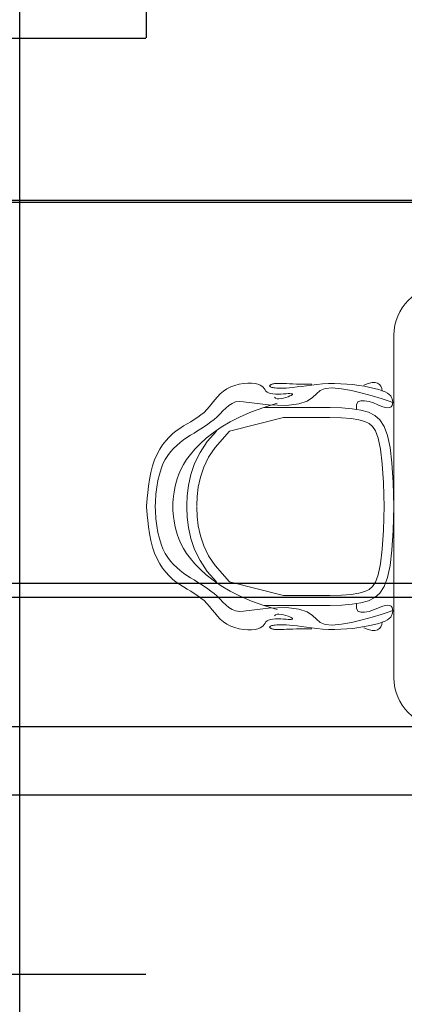
# Model space of a CAD drawing. Units: inches. Extents: x 1454 to 2136, y 626 to 1213.
# Tile 7 of 23: x 1561 to 1592, y 1062 to 1141. Entities that reach past the tile are written whole.
import ezdxf

# ---------------------------------------------------------------- set-up
doc = ezdxf.new("R2010")
doc.units = ezdxf.units.IN
doc.header["$MEASUREMENT"] = 0
for name, color, linetype, lineweight in [('A-ANNO-DIMS', 2, 'Continuous', 18), ('A-FURN-PATT', 252, 'Continuous', 13), ('conference', 41, 'Continuous', 18)]:
    doc.layers.add(name, color=color, linetype=linetype, lineweight=lineweight)
doc.styles.get("Standard").update_dxf_attribs({"font": 'arial.ttf'})
doc.dimstyles.get("Standard").update_dxf_attribs({"dimtxt": 4, "dimasz": 0.18, "dimexe": 0.18, "dimexo": 0.0625, "dimgap": 0.09, "dimtad": 0, "dimtih": 1, "dimtoh": 1, "dimdec": 0, "dimrnd": 6, "dimzin": 0, "dimdsep": 46, "dimlunit": 3, "dimtxsty": 'Standard', "dimcen": 0.09, "dimadec": 0, "dimazin": 0, "dimtfac": 1, "dimtdec": 0, "dimtofl": 0, "dimtmove": 0, "dimatfit": 3, "dimfxl": 1, "dimtolj": 1, "dimtzin": 0, "dimarcsym": 0})

# ---------------------------------------------------------------- blocks, each defined once
blk = doc.blocks.new('ОГ52_на12персон_стол2800х900')
for p, q in [((-1400, 179.3), (-1400, -520.7)), ((-1698.8, 81.1), (-1707.3, 80.4)), ((-1690.9, 81.1), (-1698.8, 81.1)), ((-1683.8, 80.4), (-1690.9, 81.1)), ((-1643.8, 80.2), (-1641.7, 80.4)), ((-1641.7, 80.4), (-1639.2, 80.6)), ((-1639.2, 80.6), (-1636.3, 80.7)), ((-1636.3, 80.7), (-1633, 80.7)), ((-1633, 80.7), (-1629.1, 80.6)), ((-1629.1, 80.6), (-1624.7, 80.4)), ((-1461.7, 77.3), (-1452.5, 80.6)), ((-1452.5, 80.6), (-1444.8, 82.3)), ((-1444.8, 82.3), (-1438.5, 82.4)), ((-1438.5, 82.4), (-1433.5, 81.2)), ((-1433.5, 81.2), (-1429.7, 78.7)), ((-1748.4, 64.9), (-1754.8, 59.3)), ((-1741.3, 69.7), (-1748.4, 64.9)), ((-1733.4, 73.6), (-1741.3, 69.7)), ((-1724.9, 76.7), (-1733.4, 73.6)), ((-1716.1, 78.9), (-1724.9, 76.7)), ((-1707.3, 80.4), (-1716.1, 78.9)), ((-1677.9, 79.2), (-1683.8, 80.4)), ((-1673.4, 77.4), (-1677.9, 79.2)), ((-1669.9, 75.2), (-1673.4, 77.4)), ((-1667.4, 72.7), (-1669.9, 75.2)), ((-1665.3, 70.1), (-1667.4, 72.7)), ((-1663.4, 67.5), (-1665.3, 70.1)), ((-1661.5, 65), (-1663.4, 67.5)), ((-1659.2, 62.9), (-1661.5, 65)), ((-1656.2, 61.1), (-1659.2, 62.9)), ((-1652.2, 59.9), (-1656.2, 61.1)), ((-1654, 75.6), (-1653.9, 76.2)), ((-1653.9, 75.1), (-1654, 75.6)), ((-1653.9, 76.2), (-1653.6, 76.6)), ((-1653.6, 74.6), (-1653.9, 75.1)), ((-1653.6, 76.6), (-1653.2, 77.1)), ((-1653, 74.1), (-1653.6, 74.6)), ((-1653.2, 77.1), (-1652.6, 77.6)), ((-1652.2, 73.6), (-1653, 74.1)), ((-1652.6, 77.6), (-1651.8, 78)), ((-1651, 73.1), (-1652.2, 73.6)), ((-1651.8, 78), (-1650.9, 78.4)), ((-1649.5, 72.6), (-1651, 73.1)), ((-1650.9, 78.4), (-1649.8, 78.9)), ((-1649.8, 78.9), (-1648.6, 79.2)), ((-1647.6, 72.1), (-1649.5, 72.6)), ((-1648.6, 79.2), (-1647.2, 79.6)), ((-1645.3, 71.7), (-1647.6, 72.1)), ((-1647.2, 79.6), (-1645.6, 79.9)), ((-1645.6, 79.9), (-1643.8, 80.2)), ((-1642.6, 71.3), (-1645.3, 71.7)), ((-1639.4, 71), (-1642.6, 71.3)), ((-1635.6, 70.7), (-1639.4, 71)), ((-1631.2, 70.7), (-1635.6, 70.7)), ((-1626.1, 70.7), (-1631.2, 70.7)), ((-1620.3, 71), (-1626.1, 70.7)), ((-1624.7, 80.4), (-1619.6, 80.2)), ((-1613.7, 71.5), (-1620.3, 71)), ((-1619.6, 80.2), (-1613.7, 79.9)), ((-1613.7, 79.9), (-1606.8, 79.6)), ((-1606.3, 72.3), (-1613.7, 71.5)), ((-1606.8, 79.6), (-1598.9, 79.4)), ((-1598, 73.4), (-1606.3, 72.3)), ((-1598.9, 79.4), (-1589.9, 79.2)), ((-1588.9, 74.6), (-1598, 73.4)), ((-1589.9, 79.2), (-1579.5, 79.2)), ((-1579, 76), (-1588.9, 74.6)), ((-1579.5, 79.2), (-1567.8, 79.4)), ((-1568.5, 77.3), (-1579, 76)), ((-1557.4, 78.6), (-1568.5, 77.3)), ((-1558.5, 59.6), (-1550.8, 66.2)), ((-1545.8, 79.5), (-1557.4, 78.6)), ((-1550.8, 66.2), (-1540.7, 70.5)), ((-1533.8, 80.2), (-1545.8, 79.5)), ((-1540.7, 70.5), (-1526, 71.6)), ((-1521.4, 80.4), (-1533.8, 80.2)), ((-1526, 71.6), (-1507.4, 69.8)), ((-1508.8, 80.1), (-1521.4, 80.4)), ((-1496.2, 79.3), (-1508.8, 80.1)), ((-1507.4, 69.8), (-1486.6, 66)), ((-1483.7, 78.1), (-1496.2, 79.3)), ((-1486.6, 66), (-1465.2, 60.9)), ((-1471.6, 76.5), (-1483.7, 78.1)), ((-1460.1, 74.7), (-1471.6, 76.5)), ((-1465.2, 60.9), (-1444.5, 55.2)), ((-1449.3, 72.6), (-1460.1, 74.7)), ((-1439.6, 70.4), (-1449.3, 72.6)), ((-1431, 68), (-1439.6, 70.4)), ((-1423.8, 65.6), (-1431, 68)), ((-1429.7, 78.7), (-1426.9, 75.1)), ((-1426.9, 75.1), (-1425, 70.5)), ((-1425, 70.5), (-1423.8, 65)), ((-1417.9, 63.2), (-1423.8, 65.6)), ((-1413.2, 60.6), (-1417.9, 63.2)), ((-1409.5, 58), (-1413.2, 60.6)), ((-1766.3, 46.8), (-1771.6, 40.2)), ((-1760.7, 53.2), (-1766.3, 46.8)), ((-1754.8, 59.3), (-1760.7, 53.2)), ((-1723.6, 42.7), (-1730.7, 39.8)), ((-1715.9, 43.9), (-1723.6, 42.7)), ((-1707.2, 43.1), (-1715.9, 43.9)), ((-1707.2, 43.1), (-1656.2, 36.7)), ((-1647.5, 59.2), (-1652.2, 59.9)), ((-1642.2, 58.9), (-1647.5, 59.2)), ((-1644.1, 52.8), (-1642.1, 50.6)), ((-1636.6, 58.9), (-1642.2, 58.9)), ((-1642.1, 50.6), (-1638.9, 49.4)), ((-1638.9, 49.4), (-1634.9, 49.2)), ((-1631, 59), (-1636.6, 58.9)), ((-1634.9, 49.2), (-1630.3, 49.7)), ((-1625.5, 59.3), (-1631, 59)), ((-1630.3, 49.7), (-1625.5, 50.7)), ((-1620.5, 59.6), (-1625.5, 59.3)), ((-1625.5, 50.7), (-1620.8, 52)), ((-1620.8, 52), (-1616.4, 53.5)), ((-1616.1, 59.8), (-1620.5, 59.6)), ((-1616.4, 53.5), (-1612.7, 55)), ((-1612.5, 59.9), (-1616.1, 59.8)), ((-1612.7, 55), (-1609.9, 56.3)), ((-1609.8, 59.7), (-1612.5, 59.9)), ((-1609.9, 56.3), (-1608, 57.4)), ((-1608, 59.4), (-1609.8, 59.7)), ((-1607.1, 58.9), (-1608, 59.4)), ((-1608, 57.4), (-1607.1, 58.2)), ((-1607.1, 58.2), (-1607.1, 58.9)), ((-1594.1, 38.7), (-1577.3, 44.6)), ((-1577.3, 44.6), (-1566.4, 51.9)), ((-1566.4, 51.9), (-1558.5, 59.6)), ((-1473.6, 42.8), (-1476.8, 37.1)), ((-1467.8, 45.4), (-1473.6, 42.8)), ((-1460, 45.4), (-1467.8, 45.4)), ((-1451, 43.6), (-1460, 45.4)), ((-1441.6, 40.7), (-1451, 43.6)), ((-1444.5, 55.2), (-1426.1, 49.6)), ((-1432.7, 37.2), (-1441.6, 40.7)), ((-1426.1, 49.6), (-1411.6, 44.9)), ((-1411.6, 44.9), (-1402.6, 41.8)), ((-1406.7, 55.2), (-1409.5, 58)), ((-1404.8, 52.2), (-1406.7, 55.2)), ((-1403.5, 49.1), (-1404.8, 52.2)), ((-1402.8, 45.8), (-1403.5, 49.1)), ((-1402.9, 38.8), (-1402.5, 42.3)), ((-1402.5, 42.3), (-1402.8, 45.8)), ((-1788.1, 21.5), (-1794.4, 16.2)), ((-1782.4, 27.4), (-1788.1, 21.5)), ((-1776.9, 33.7), (-1782.4, 27.4)), ((-1771.6, 40.2), (-1776.9, 33.7)), ((-1749.4, 24.7), (-1755.3, 18.6)), ((-1743.5, 30.4), (-1749.4, 24.7)), ((-1737.3, 35.6), (-1743.5, 30.4)), ((-1730.7, 39.8), (-1737.3, 35.6)), ((-1691.4, 22.5), (-1714.2, 12.5)), ((-1666.1, 31.7), (-1691.4, 22.5)), ((-1638.3, 40), (-1666.1, 31.7)), ((-1666.1, 31.7), (-1625.8, 31.2)), ((-1656.2, 36.7), (-1619.4, 35.7)), ((-1625.8, 31.2), (-1589.9, 31.2)), ((-1619.4, 35.7), (-1594.1, 38.7)), ((-1589.9, 31.2), (-1558.2, 31.3)), ((-1558.2, 31.3), (-1530.4, 31.2)), ((-1530.4, 31.2), (-1506.3, 30.5)), ((-1506.3, 30.5), (-1485.4, 29)), ((-1485.4, 29), (-1467.4, 26.2)), ((-1476.8, 37.1), (-1476.4, 27.6)), ((-1467.4, 26.2), (-1452.2, 21.8)), ((-1452.2, 21.8), (-1439.4, 15.4)), ((-1424.9, 33.8), (-1432.7, 37.2)), ((-1424.9, 33.8), (-1418.1, 31.4)), ((-1418.1, 31.4), (-1412.8, 30.6)), ((-1412.8, 30.6), (-1408.7, 31.2)), ((-1408.7, 31.2), (-1405.8, 33)), ((-1405.8, 33), (-1403.9, 35.6)), ((-1403.9, 35.6), (-1402.9, 38.8)), ((-1815.2, 2.5), (-1822.6, -1.8)), ((-1808, 6.9), (-1815.2, 2.5)), ((-1801, 11.4), (-1808, 6.9)), ((-1794.4, 16.2), (-1801, 11.4)), ((-1773.9, 2.1), (-1780.6, -2.8)), ((-1767.5, 7.2), (-1773.9, 2.1)), ((-1761.3, 12.7), (-1767.5, 7.2)), ((-1755.3, 18.6), (-1761.3, 12.7)), ((-1734.8, 2), (-1753.1, -8.9)), ((-1735.7, -17.1), (-1625.9, 11.2)), ((-1714.2, 12.5), (-1734.8, 2)), ((-1625.9, 11.2), (-1589.9, 11.2)), ((-1589.9, 11.2), (-1558.2, 11.3)), ((-1558.2, 11.3), (-1530.8, 11.2)), ((-1530.8, 11.2), (-1507.3, 10.5)), ((-1507.3, 10.5), (-1487.6, 9.1)), ((-1487.6, 9.1), (-1471.7, 6.6)), ((-1471.7, 6.6), (-1459.5, 3.1)), ((-1459.5, 3.1), (-1450.6, -1.3)), ((-1439.4, 15.4), (-1428.7, 6.1)), ((-1428.7, 6.1), (-1420.1, -7.2)), ((-1845, -16.4), (-1852.3, -22.3)), ((-1837.6, -11.1), (-1845, -16.4)), ((-1830.1, -6.3), (-1837.6, -11.1)), ((-1822.6, -1.8), (-1830.1, -6.3)), ((-1801.4, -16.3), (-1808.5, -20.7)), ((-1794.3, -11.8), (-1801.4, -16.3)), ((-1787.4, -7.4), (-1794.3, -11.8)), ((-1780.6, -2.8), (-1787.4, -7.4)), ((-1769.4, -20.1), (-1783.7, -31.3)), ((-1762.3, -16.7), (-1781.4, -38.1)), ((-1753.1, -8.9), (-1769.4, -20.1)), ((-1735.7, -17.1), (-1765.6, -50.4)), ((-1450.6, -1.3), (-1444, -7.1)), ((-1444, -7.1), (-1438, -16.3)), ((-1438, -16.3), (-1432.5, -31.2)), ((-1420.1, -7.2), (-1413.2, -25.6)), ((-1866.2, -36.3), (-1872.7, -44.6)), ((-1859.4, -29), (-1866.2, -36.3)), ((-1852.3, -22.3), (-1859.4, -29)), ((-1837, -40.2), (-1843.8, -45.9)), ((-1830, -34.9), (-1837, -40.2)), ((-1822.9, -29.9), (-1830, -34.9)), ((-1815.7, -25.2), (-1822.9, -29.9)), ((-1808.5, -20.7), (-1815.7, -25.2)), ((-1781.4, -38.1), (-1796.2, -60.3)), ((-1783.7, -31.3), (-1796.1, -42.5)), ((-1432.5, -31.2), (-1427.7, -53.4)), ((-1413.2, -25.6), (-1408, -50.1)), ((-1878.7, -53.8), (-1884.1, -64)), ((-1872.7, -44.6), (-1878.7, -53.8)), ((-1856.4, -59), (-1862.1, -66.5)), ((-1850.3, -52.2), (-1856.4, -59)), ((-1843.8, -45.9), (-1850.3, -52.2)), ((-1806.8, -53.5), (-1816, -64.2)), ((-1796.2, -60.3), (-1807.2, -82.9)), ((-1796.1, -42.5), (-1806.8, -53.5)), ((-1765.6, -50.4), (-1778.8, -70.2)), ((-1427.7, -53.4), (-1424.1, -83.6)), ((-1408, -50.1), (-1404.2, -81.7)), ((-1889, -75.2), (-1893.2, -87.7)), ((-1884.1, -64), (-1889, -75.2)), ((-1867.3, -74.8), (-1871.9, -83.9)), ((-1862.1, -66.5), (-1867.3, -74.8)), ((-1823.7, -74.7), (-1830.1, -84.9)), ((-1816, -64.2), (-1823.7, -74.7)), ((-1778.8, -70.2), (-1788.7, -90.5)), ((-1893.2, -87.7), (-1896.7, -101.2)), ((-1875.9, -94), (-1879.3, -105.1)), ((-1871.9, -83.9), (-1875.9, -94)), ((-1835.3, -94.9), (-1839.6, -104.7)), ((-1830.1, -84.9), (-1835.3, -94.9)), ((-1807.2, -82.9), (-1814.8, -105.5)), ((-1788.7, -90.5), (-1795.5, -110.8)), ((-1424.1, -83.6), (-1421.5, -122.5)), ((-1404.2, -81.7), (-1401.6, -121.6)), ((-1899.4, -115.3), (-1901.6, -129.2)), ((-1896.7, -101.2), (-1899.4, -115.3)), ((-1882.2, -117.4), (-1884.5, -130.9)), ((-1879.3, -105.1), (-1882.2, -117.4)), ((-1843, -114.3), (-1845.6, -123.7)), ((-1839.6, -104.7), (-1843, -114.3)), ((-1814.8, -105.5), (-1819.7, -127.5)), ((-1795.5, -110.8), (-1800, -130.9)), ((-1901.6, -129.2), (-1903.2, -142.1)), ((-1884.5, -130.9), (-1886.2, -145.8)), ((-1847.7, -132.7), (-1849.2, -141.4)), ((-1845.6, -123.7), (-1847.7, -132.7)), ((-1819.7, -127.5), (-1822.3, -148.6)), ((-1800, -130.9), (-1802.3, -150.3)), ((-1421.5, -122.5), (-1420, -171.3)), ((-1401.6, -121.6), (-1400, -170.7)), ((-1904.4, -153.5), (-1905.1, -162.5)), ((-1903.2, -142.1), (-1904.4, -153.5)), ((-1886.2, -145.8), (-1887.4, -162.1)), ((-1851, -156.4), (-1851.5, -162.3)), ((-1850.3, -149.3), (-1851, -156.4)), ((-1849.2, -141.4), (-1850.3, -149.3)), ((-1822.3, -148.6), (-1823.1, -168.3)), ((-1802.3, -150.3), (-1803.1, -168.6)), ((-1905.5, -168.5), (-1905.7, -170.7)), ((-1905.5, -172.9), (-1905.7, -170.7)), ((-1905.1, -162.5), (-1905.5, -168.5)), ((-1905.1, -178.9), (-1905.5, -172.9)), ((-1904.4, -187.9), (-1905.1, -178.9)), ((-1887.4, -162.1), (-1887.8, -170.7)), ((-1887.4, -179.3), (-1887.8, -170.7)), ((-1886.2, -195.6), (-1887.4, -179.3)), ((-1851.7, -166.8), (-1851.8, -169.6)), ((-1851.8, -169.6), (-1851.8, -170.7)), ((-1851.8, -171.7), (-1851.8, -170.7)), ((-1851.7, -174.6), (-1851.8, -171.7)), ((-1851.5, -162.3), (-1851.7, -166.8)), ((-1851.5, -179.1), (-1851.7, -174.6)), ((-1851, -185), (-1851.5, -179.1)), ((-1823.1, -168.3), (-1823.1, -170.7)), ((-1823.1, -173), (-1823.1, -170.7)), ((-1822.3, -192.7), (-1823.1, -173)), ((-1803.1, -168.6), (-1803.1, -170.3)), ((-1803.1, -172.8), (-1803.1, -171.1)), ((-1802.3, -191.1), (-1803.1, -172.8)), ((-1421.5, -218.8), (-1420, -170)), ((-1401.6, -219.8), (-1400, -170.7)), ((-1903.2, -199.2), (-1904.4, -187.9)), ((-1901.6, -212.2), (-1903.2, -199.2)), ((-1884.5, -210.5), (-1886.2, -195.6)), ((-1850.3, -192), (-1851, -185)), ((-1849.2, -200), (-1850.3, -192)), ((-1847.7, -208.6), (-1849.2, -200)), ((-1819.7, -213.8), (-1822.3, -192.7)), ((-1800, -210.5), (-1802.3, -191.1)), ((-1899.4, -226.1), (-1901.6, -212.2)), ((-1882.2, -224), (-1884.5, -210.5)), ((-1845.6, -217.7), (-1847.7, -208.6)), ((-1843, -227), (-1845.6, -217.7)), ((-1814.8, -235.9), (-1819.7, -213.8)), ((-1795.5, -230.5), (-1800, -210.5)), ((-1424.1, -257.8), (-1421.5, -218.8)), ((-1404.2, -259.6), (-1401.6, -219.8)), ((-1896.7, -240.1), (-1899.4, -226.1)), ((-1893.2, -253.7), (-1896.7, -240.1)), ((-1879.3, -236.2), (-1882.2, -224)), ((-1875.9, -247.3), (-1879.3, -236.2)), ((-1839.6, -236.6), (-1843, -227)), ((-1835.3, -246.4), (-1839.6, -236.6)), ((-1807.2, -258.5), (-1814.8, -235.9)), ((-1788.7, -250.9), (-1795.5, -230.5)), ((-1889, -266.1), (-1893.2, -253.7)), ((-1871.9, -257.4), (-1875.9, -247.3)), ((-1867.3, -266.5), (-1871.9, -257.4)), ((-1830.1, -256.4), (-1835.3, -246.4)), ((-1823.7, -266.7), (-1830.1, -256.4)), ((-1796.2, -281.1), (-1807.2, -258.5)), ((-1778.8, -271.1), (-1788.7, -250.9)), ((-1427.7, -288), (-1424.1, -257.8)), ((-1408, -291.3), (-1404.2, -259.6)), ((-1884.1, -277.4), (-1889, -266.1)), ((-1878.7, -287.6), (-1884.1, -277.4)), ((-1862.1, -274.8), (-1867.3, -266.5)), ((-1856.4, -282.3), (-1862.1, -274.8)), ((-1816, -277.2), (-1823.7, -266.7)), ((-1806.8, -287.9), (-1816, -277.2)), ((-1781.4, -303.3), (-1796.2, -281.1)), ((-1765.6, -291), (-1778.8, -271.1)), ((-1872.7, -296.8), (-1878.7, -287.6)), ((-1866.2, -305), (-1872.7, -296.8)), ((-1850.3, -289.2), (-1856.4, -282.3)), ((-1843.8, -295.4), (-1850.3, -289.2)), ((-1837, -301.2), (-1843.8, -295.4)), ((-1830, -306.5), (-1837, -301.2)), ((-1796.1, -298.9), (-1806.8, -287.9)), ((-1783.7, -310), (-1796.1, -298.9)), ((-1735.7, -324.3), (-1765.6, -291)), ((-1432.5, -310.2), (-1427.7, -288)), ((-1413.2, -315.8), (-1408, -291.3)), ((-1859.4, -312.4), (-1866.2, -305)), ((-1852.3, -319), (-1859.4, -312.4)), ((-1845, -324.9), (-1852.3, -319)), ((-1822.9, -311.4), (-1830, -306.5)), ((-1815.7, -316.1), (-1822.9, -311.4)), ((-1808.5, -320.7), (-1815.7, -316.1)), ((-1801.4, -325.1), (-1808.5, -320.7)), ((-1769.4, -321.3), (-1783.7, -310)), ((-1762.3, -324.6), (-1781.4, -303.3)), ((-1753.1, -332.5), (-1769.4, -321.3)), ((-1438, -325.1), (-1432.5, -310.2)), ((-1420.1, -334.1), (-1413.2, -315.8)), ((-1837.6, -330.2), (-1845, -324.9)), ((-1830.1, -335), (-1837.6, -330.2)), ((-1822.6, -339.5), (-1830.1, -335)), ((-1815.2, -343.9), (-1822.6, -339.5)), ((-1794.3, -329.5), (-1801.4, -325.1)), ((-1787.4, -334), (-1794.3, -329.5)), ((-1780.6, -338.6), (-1787.4, -334)), ((-1773.9, -343.4), (-1780.6, -338.6)), ((-1734.8, -343.4), (-1753.1, -332.5)), ((-1735.7, -324.3), (-1625.9, -352.6)), ((-1459.5, -344.4), (-1450.6, -340)), ((-1450.6, -340), (-1444, -334.2)), ((-1444, -334.2), (-1438, -325.1)), ((-1428.7, -347.5), (-1420.1, -334.1)), ((-1808, -348.2), (-1815.2, -343.9)), ((-1801, -352.8), (-1808, -348.2)), ((-1794.4, -357.6), (-1801, -352.8)), ((-1788.1, -362.9), (-1794.4, -357.6)), ((-1767.5, -348.6), (-1773.9, -343.4)), ((-1761.3, -354.1), (-1767.5, -348.6)), ((-1755.3, -360), (-1761.3, -354.1)), ((-1749.4, -366), (-1755.3, -360)), ((-1714.2, -353.9), (-1734.8, -343.4)), ((-1691.4, -363.8), (-1714.2, -353.9)), ((-1625.9, -352.6), (-1589.9, -352.6)), ((-1589.9, -352.6), (-1558.2, -352.7)), ((-1558.2, -352.7), (-1530.8, -352.6)), ((-1530.8, -352.6), (-1507.3, -351.9)), ((-1507.3, -351.9), (-1487.6, -350.4)), ((-1487.6, -350.4), (-1471.7, -348)), ((-1471.7, -348), (-1459.5, -344.4)), ((-1452.2, -363.2), (-1439.4, -356.8)), ((-1439.4, -356.8), (-1428.7, -347.5)), ((-1782.4, -368.7), (-1788.1, -362.9)), ((-1776.9, -375), (-1782.4, -368.7)), ((-1771.6, -381.6), (-1776.9, -375)), ((-1766.3, -388.1), (-1771.6, -381.6)), ((-1743.5, -371.8), (-1749.4, -366)), ((-1737.3, -376.9), (-1743.5, -371.8)), ((-1730.7, -381.1), (-1737.3, -376.9)), ((-1723.6, -384), (-1730.7, -381.1)), ((-1707.2, -384.5), (-1656.2, -378.1)), ((-1666.1, -373), (-1691.4, -363.8)), ((-1666.1, -373), (-1625.8, -372.6)), ((-1638.3, -381.3), (-1666.1, -373)), ((-1656.2, -378.1), (-1619.4, -377.1)), ((-1625.8, -372.6), (-1589.9, -372.6)), ((-1619.4, -377.1), (-1594.1, -380.1)), ((-1594.1, -380.1), (-1577.3, -385.9)), ((-1589.9, -372.6), (-1558.2, -372.7)), ((-1558.2, -372.7), (-1530.4, -372.6)), ((-1530.4, -372.6), (-1506.3, -371.9)), ((-1506.3, -371.9), (-1485.4, -370.3)), ((-1485.4, -370.3), (-1467.4, -367.5)), ((-1476.8, -378.4), (-1476.4, -368.9)), ((-1473.6, -384.2), (-1476.8, -378.4)), ((-1467.4, -367.5), (-1452.2, -363.2)), ((-1432.7, -378.5), (-1441.6, -382)), ((-1424.9, -375.1), (-1432.7, -378.5)), ((-1424.9, -375.1), (-1418.1, -372.7)), ((-1418.1, -372.7), (-1412.8, -372)), ((-1412.8, -372), (-1408.7, -372.6)), ((-1408.7, -372.6), (-1405.8, -374.3)), ((-1405.8, -374.3), (-1403.9, -376.9)), ((-1403.9, -376.9), (-1402.9, -380.1)), ((-1402.9, -380.1), (-1402.5, -383.6)), ((-1760.7, -394.6), (-1766.3, -388.1)), ((-1754.8, -400.7), (-1760.7, -394.6)), ((-1748.4, -406.2), (-1754.8, -400.7)), ((-1715.9, -385.3), (-1723.6, -384)), ((-1707.2, -384.5), (-1715.9, -385.3)), ((-1652.2, -401.3), (-1656.2, -402.5)), ((-1647.5, -400.6), (-1652.2, -401.3)), ((-1642.2, -400.3), (-1647.5, -400.6)), ((-1644.1, -394.1), (-1642.1, -391.9)), ((-1636.6, -400.2), (-1642.2, -400.3)), ((-1642.1, -391.9), (-1638.9, -390.8)), ((-1638.9, -390.8), (-1634.9, -390.6)), ((-1631, -400.4), (-1636.6, -400.2)), ((-1634.9, -390.6), (-1630.3, -391.1)), ((-1625.5, -400.7), (-1631, -400.4)), ((-1630.3, -391.1), (-1625.5, -392)), ((-1625.5, -392), (-1620.8, -393.4)), ((-1620.5, -401), (-1625.5, -400.7)), ((-1620.8, -393.4), (-1616.4, -394.9)), ((-1616.1, -401.2), (-1620.5, -401)), ((-1616.4, -394.9), (-1612.7, -396.3)), ((-1612.5, -401.2), (-1616.1, -401.2)), ((-1612.7, -396.3), (-1609.9, -397.6)), ((-1609.8, -401.1), (-1612.5, -401.2)), ((-1609.9, -397.6), (-1608, -398.7)), ((-1608, -400.8), (-1609.8, -401.1)), ((-1608, -398.7), (-1607.1, -399.6)), ((-1607.1, -400.3), (-1608, -400.8)), ((-1607.1, -399.6), (-1607.1, -400.3)), ((-1577.3, -385.9), (-1566.4, -393.3)), ((-1566.4, -393.3), (-1558.5, -400.9)), ((-1558.5, -400.9), (-1550.8, -407.5)), ((-1467.8, -386.7), (-1473.6, -384.2)), ((-1460, -386.8), (-1467.8, -386.7)), ((-1465.2, -402.3), (-1444.5, -396.5)), ((-1451, -385), (-1460, -386.8)), ((-1441.6, -382), (-1451, -385)), ((-1444.5, -396.5), (-1426.1, -391)), ((-1426.1, -391), (-1411.6, -386.3)), ((-1413.2, -402), (-1417.9, -404.5)), ((-1409.5, -399.3), (-1413.2, -402)), ((-1411.6, -386.3), (-1402.6, -383.2)), ((-1406.7, -396.6), (-1409.5, -399.3)), ((-1404.8, -393.6), (-1406.7, -396.6)), ((-1403.5, -390.5), (-1404.8, -393.6)), ((-1402.8, -387.1), (-1403.5, -390.5)), ((-1402.5, -383.6), (-1402.8, -387.1)), ((-1741.3, -411), (-1748.4, -406.2)), ((-1733.4, -415), (-1741.3, -411)), ((-1724.9, -418), (-1733.4, -415)), ((-1716.1, -420.3), (-1724.9, -418)), ((-1707.3, -421.7), (-1716.1, -420.3)), ((-1698.8, -422.4), (-1707.3, -421.7)), ((-1683.8, -421.8), (-1690.9, -422.4)), ((-1677.9, -420.5), (-1683.8, -421.8)), ((-1673.4, -418.7), (-1677.9, -420.5)), ((-1669.9, -416.5), (-1673.4, -418.7)), ((-1667.4, -414.1), (-1669.9, -416.5)), ((-1665.3, -411.4), (-1667.4, -414.1)), ((-1663.4, -408.8), (-1665.3, -411.4)), ((-1661.5, -406.4), (-1663.4, -408.8)), ((-1659.2, -404.2), (-1661.5, -406.4)), ((-1656.2, -402.5), (-1659.2, -404.2)), ((-1653.9, -416.5), (-1654, -417)), ((-1654, -417), (-1653.9, -417.5)), ((-1653.6, -416), (-1653.9, -416.5)), ((-1653.9, -417.5), (-1653.6, -418)), ((-1653, -415.4), (-1653.6, -416)), ((-1653.6, -418), (-1653.2, -418.5)), ((-1653.2, -418.5), (-1652.6, -418.9)), ((-1652.2, -414.9), (-1653, -415.4)), ((-1652.6, -418.9), (-1651.8, -419.4)), ((-1651, -414.4), (-1652.2, -414.9)), ((-1651.8, -419.4), (-1650.9, -419.8)), ((-1649.5, -413.9), (-1651, -414.4)), ((-1650.9, -419.8), (-1649.8, -420.2)), ((-1649.8, -420.2), (-1648.6, -420.6)), ((-1647.6, -413.5), (-1649.5, -413.9)), ((-1648.6, -420.6), (-1647.2, -421)), ((-1645.3, -413), (-1647.6, -413.5)), ((-1647.2, -421), (-1645.6, -421.3)), ((-1645.6, -421.3), (-1643.8, -421.6)), ((-1642.6, -412.7), (-1645.3, -413)), ((-1643.8, -421.6), (-1641.7, -421.8)), ((-1639.4, -412.3), (-1642.6, -412.7)), ((-1641.7, -421.8), (-1639.2, -422)), ((-1635.6, -412.1), (-1639.4, -412.3)), ((-1639.2, -422), (-1636.3, -422)), ((-1636.3, -422), (-1633, -422)), ((-1631.2, -412), (-1635.6, -412.1)), ((-1633, -422), (-1629.1, -422)), ((-1626.1, -412.1), (-1631.2, -412)), ((-1629.1, -422), (-1624.7, -421.8)), ((-1620.3, -412.4), (-1626.1, -412.1)), ((-1624.7, -421.8), (-1619.6, -421.5)), ((-1613.7, -412.9), (-1620.3, -412.4)), ((-1619.6, -421.5), (-1613.7, -421.2)), ((-1606.3, -413.7), (-1613.7, -412.9)), ((-1613.7, -421.2), (-1606.8, -421)), ((-1606.8, -421), (-1598.9, -420.7)), ((-1598, -414.7), (-1606.3, -413.7)), ((-1598.9, -420.7), (-1589.9, -420.6)), ((-1588.9, -416), (-1598, -414.7)), ((-1589.9, -420.6), (-1579.5, -420.6)), ((-1579, -417.4), (-1588.9, -416)), ((-1579.5, -420.6), (-1567.8, -420.7)), ((-1568.5, -418.7), (-1579, -417.4)), ((-1557.4, -419.9), (-1568.5, -418.7)), ((-1545.8, -420.9), (-1557.4, -419.9)), ((-1550.8, -407.5), (-1540.7, -411.8)), ((-1533.8, -421.6), (-1545.8, -420.9)), ((-1540.7, -411.8), (-1526, -412.9)), ((-1521.4, -421.8), (-1533.8, -421.6)), ((-1526, -412.9), (-1507.4, -411.2)), ((-1508.8, -421.5), (-1521.4, -421.8)), ((-1496.2, -420.7), (-1508.8, -421.5)), ((-1507.4, -411.2), (-1486.6, -407.4)), ((-1483.7, -419.5), (-1496.2, -420.7)), ((-1486.6, -407.4), (-1465.2, -402.3)), ((-1471.6, -417.9), (-1483.7, -419.5)), ((-1460.1, -416), (-1471.6, -417.9)), ((-1461.7, -418.7), (-1452.5, -422)), ((-1449.3, -414), (-1460.1, -416)), ((-1452.5, -422), (-1444.8, -423.7)), ((-1439.6, -411.7), (-1449.3, -414)), ((-1431, -409.4), (-1439.6, -411.7)), ((-1433.5, -422.6), (-1429.7, -420.1)), ((-1423.8, -407), (-1431, -409.4)), ((-1429.7, -420.1), (-1426.9, -416.5)), ((-1426.9, -416.5), (-1425, -411.9)), ((-1425, -411.9), (-1423.8, -406.4)), ((-1417.9, -404.5), (-1423.8, -407)), ((-1690.9, -422.4), (-1698.8, -422.4)), ((-1444.8, -423.7), (-1438.5, -423.8)), ((-1438.5, -423.8), (-1433.5, -422.6))]:
    blk.add_line(p, q)
for centre, start, end in [((-1300, 179.3), 90, 180), ((-1300, -520.7), 180, 270)]:
    blk.add_arc(centre, 100, start, end)
blk = doc.blocks.new('*D23')
at = {"layer": 'A-ANNO-DIMS', "color": 0, "lineweight": -2, "transparency": 16777216}
for p, q in [((1571.674, 1139.532), (1571.674, 1162.157)), ((1721.725, 1139.532), (1721.725, 1162.157)), ((1571.854, 1161.977), (1615.675, 1161.977)), ((1721.545, 1161.977), (1677.724, 1161.977))]:
    blk.add_line(p, q, dxfattribs=at)
at = {"layer": 'A-ANNO-DIMS', "color": 0, "transparency": 16777216}
for points in [[(1571.854, 1162.007), (1571.854, 1161.947), (1571.674, 1161.977)], [(1721.545, 1162.007), (1721.545, 1161.947), (1721.725, 1161.977)]]:
    blk.add_solid(points, dxfattribs=at)
at = {"layer": 'Defpoints', "color": 0, "transparency": 16777216}
for p in [(1721.725, 1161.977), (1571.674, 1139.469), (1721.725, 1139.469)]:
    blk.add_point(p, dxfattribs=at)
at = {"layer": 'A-ANNO-DIMS', "color": 0, "transparency": 16777216, "insert": (1646.7, 1161.977), "char_height": 4, "attachment_point": 5}
blk.add_mtext('\\A1;CONFERENCE SET 150', dxfattribs=at)
blk = doc.blocks.new('*D24')
at = {"layer": 'A-ANNO-DIMS', "color": 0, "lineweight": -2, "transparency": 16777216}
for p, q in [((1571.612, 1139.469), (1548.986, 1139.469)), ((1549.166, 1139.289), (1549.166, 1103.969)), ((1549.166, 1064.401), (1549.166, 1099.721)), ((1571.612, 1064.221), (1548.986, 1064.221))]:
    blk.add_line(p, q, dxfattribs=at)
at = {"layer": 'A-ANNO-DIMS', "color": 0, "transparency": 16777216}
for points in [[(1549.136, 1139.289), (1549.196, 1139.289), (1549.166, 1139.469)], [(1549.136, 1064.401), (1549.196, 1064.401), (1549.166, 1064.221)]]:
    blk.add_solid(points, dxfattribs=at)
at = {"layer": 'Defpoints', "color": 0, "transparency": 16777216}
for p in [(1549.166, 1139.469), (1571.674, 1139.469), (1571.674, 1064.221)]:
    blk.add_point(p, dxfattribs=at)
at = {"layer": 'A-ANNO-DIMS', "color": 0, "transparency": 16777216, "insert": (1549.166, 1101.845), "char_height": 4, "attachment_point": 5}
blk.add_mtext('\\A1;75', dxfattribs=at)
blk = doc.blocks.new('*D33')
at = {"layer": 'A-ANNO-DIMS', "color": 0, "lineweight": -2, "transparency": 16777216}
for p, q in [((2032.494, 1126.282), (1462.374, 1126.282)), ((1462.554, 1126.102), (1462.554, 1056.381)), ((1462.554, 982.462), (1462.554, 1052.184)), ((2032.494, 982.282), (1462.374, 982.282))]:
    blk.add_line(p, q, dxfattribs=at)
at = {"layer": 'A-ANNO-DIMS', "color": 0, "transparency": 16777216}
for points in [[(1462.524, 1126.102), (1462.584, 1126.102), (1462.554, 1126.282)], [(1462.524, 982.462), (1462.584, 982.462), (1462.554, 982.282)]]:
    blk.add_solid(points, dxfattribs=at)
at = {"layer": 'Defpoints', "color": 0, "transparency": 16777216}
for p in [(1462.554, 1126.282), (2032.556, 1126.282), (2032.556, 982.282)]:
    blk.add_point(p, dxfattribs=at)
at = {"layer": 'A-ANNO-DIMS', "color": 0, "transparency": 16777216, "insert": (1462.554, 1054.282), "char_height": 4, "attachment_point": 5}
blk.add_mtext('\\A1;144', dxfattribs=at)
blk = doc.blocks.new('*D40')
at = {"layer": 'A-ANNO-DIMS', "color": 0, "lineweight": -2, "transparency": 16777216}
for p, q in [((1501.556, 877.345), (1501.556, 1210.464)), ((1501.736, 1210.284), (1569.244, 1210.284)), ((1645.376, 1210.284), (1577.869, 1210.284)), ((1645.556, 877.345), (1645.556, 1210.464))]:
    blk.add_line(p, q, dxfattribs=at)
at = {"layer": 'A-ANNO-DIMS', "color": 0, "transparency": 16777216}
for points in [[(1501.736, 1210.314), (1501.736, 1210.254), (1501.556, 1210.284)], [(1645.376, 1210.314), (1645.376, 1210.254), (1645.556, 1210.284)]]:
    blk.add_solid(points, dxfattribs=at)
at = {"layer": 'Defpoints', "color": 0, "transparency": 16777216}
for p in [(1645.556, 1210.284), (1501.556, 877.282), (1645.556, 877.282)]:
    blk.add_point(p, dxfattribs=at)
at = {"layer": 'A-ANNO-DIMS', "color": 0, "transparency": 16777216, "insert": (1573.556, 1210.284), "char_height": 4, "attachment_point": 5}
blk.add_mtext('\\A1;144', dxfattribs=at)
blk = doc.blocks.new('*D54')
at = {"layer": 'A-ANNO-DIMS', "color": 0, "lineweight": -2, "transparency": 16777216}
for p, q in [((1879.494, 1126.282), (1462.374, 1126.282)), ((1462.554, 1126.102), (1462.554, 1078.915)), ((1462.554, 1027.462), (1462.554, 1074.65)), ((1879.494, 1027.282), (1462.374, 1027.282))]:
    blk.add_line(p, q, dxfattribs=at)
at = {"layer": 'A-ANNO-DIMS', "color": 0, "transparency": 16777216}
for points in [[(1462.524, 1126.102), (1462.584, 1126.102), (1462.554, 1126.282)], [(1462.524, 1027.462), (1462.584, 1027.462), (1462.554, 1027.282)]]:
    blk.add_solid(points, dxfattribs=at)
at = {"layer": 'Defpoints', "color": 0, "transparency": 16777216}
for p in [(1879.556, 1126.282), (1462.554, 1027.282), (1879.556, 1027.282)]:
    blk.add_point(p, dxfattribs=at)
at = {"layer": 'A-ANNO-DIMS', "color": 0, "transparency": 16777216, "insert": (1462.554, 1076.782), "char_height": 4, "attachment_point": 5}
blk.add_mtext('\\A1;99', dxfattribs=at)
blk = doc.blocks.new('*D55')
at = {"layer": 'A-ANNO-DIMS', "color": 0, "lineweight": -2, "transparency": 16777216}
for p, q in [((1537.556, 1018.345), (1537.556, 1210.464)), ((1537.736, 1210.284), (1542.647, 1210.284)), ((1561.304, 1210.284), (1556.393, 1210.284)), ((1561.484, 1018.345), (1561.484, 1210.464))]:
    blk.add_line(p, q, dxfattribs=at)
at = {"layer": 'A-ANNO-DIMS', "color": 0, "transparency": 16777216}
for points in [[(1537.736, 1210.314), (1537.736, 1210.254), (1537.556, 1210.284)], [(1561.304, 1210.314), (1561.304, 1210.254), (1561.484, 1210.284)]]:
    blk.add_solid(points, dxfattribs=at)
at = {"layer": 'Defpoints', "color": 0, "transparency": 16777216}
for p in [(1561.484, 1210.284), (1537.556, 1018.282), (1561.484, 1018.282)]:
    blk.add_point(p, dxfattribs=at)
at = {"layer": 'A-ANNO-DIMS', "color": 0, "transparency": 16777216, "insert": (1549.52, 1210.284), "char_height": 4, "attachment_point": 5}
blk.add_mtext('\\A1;23.93', dxfattribs=at)
blk = doc.blocks.new('*D70')
at = {"layer": 'A-ANNO-DIMS', "color": 0, "lineweight": -2, "transparency": 16777216}
for p, q in [((1811.166, 1094.525), (1462.374, 1094.525)), ((1462.554, 1094.345), (1462.554, 1088.71)), ((1462.554, 1078.811), (1462.554, 1084.445)), ((1811.166, 1078.631), (1462.374, 1078.631))]:
    blk.add_line(p, q, dxfattribs=at)
at = {"layer": 'A-ANNO-DIMS', "color": 0, "transparency": 16777216}
for points in [[(1462.524, 1094.345), (1462.584, 1094.345), (1462.554, 1094.525)], [(1462.524, 1078.811), (1462.584, 1078.811), (1462.554, 1078.631)]]:
    blk.add_solid(points, dxfattribs=at)
at = {"layer": 'Defpoints', "color": 0, "transparency": 16777216}
for p in [(1462.554, 1094.525), (1811.229, 1094.525), (1811.229, 1078.631)]:
    blk.add_point(p, dxfattribs=at)
at = {"layer": 'A-ANNO-DIMS', "color": 0, "transparency": 16777216, "insert": (1462.554, 1086.578), "char_height": 4, "attachment_point": 5}
blk.add_mtext('\\A1;15.894', dxfattribs=at)
blk = doc.blocks.new('*D73')
at = {"layer": 'A-ANNO-DIMS', "color": 0, "lineweight": -2, "transparency": 16777216}
for p, q in [((1985.096, 1126.439), (1462.374, 1126.439)), ((1462.554, 1126.259), (1462.554, 1113.178)), ((1462.554, 1095.83), (1462.554, 1108.911)), ((1966.644, 1095.65), (1462.374, 1095.65))]:
    blk.add_line(p, q, dxfattribs=at)
at = {"layer": 'A-ANNO-DIMS', "color": 0, "transparency": 16777216}
for points in [[(1462.524, 1126.259), (1462.584, 1126.259), (1462.554, 1126.439)], [(1462.524, 1095.83), (1462.584, 1095.83), (1462.554, 1095.65)]]:
    blk.add_solid(points, dxfattribs=at)
at = {"layer": 'Defpoints', "color": 0, "transparency": 16777216}
for p in [(1985.158, 1126.439), (1462.554, 1095.65), (1966.707, 1095.65)]:
    blk.add_point(p, dxfattribs=at)
at = {"layer": 'A-ANNO-DIMS', "color": 0, "transparency": 16777216, "insert": (1462.554, 1111.044), "char_height": 4, "attachment_point": 5}
blk.add_mtext('\\A1;30.79', dxfattribs=at)
blk = doc.blocks.new('*D76')
at = {"layer": 'A-ANNO-DIMS', "color": 0, "lineweight": -2, "transparency": 16777216}
for p, q in [((1962.644, 1095.65), (1462.374, 1095.65)), ((1462.554, 1095.47), (1462.554, 1073.782)), ((1462.554, 1047.83), (1462.554, 1069.517)), ((1914.644, 1047.65), (1462.374, 1047.65))]:
    blk.add_line(p, q, dxfattribs=at)
at = {"layer": 'A-ANNO-DIMS', "color": 0, "transparency": 16777216}
for points in [[(1462.524, 1095.47), (1462.584, 1095.47), (1462.554, 1095.65)], [(1462.524, 1047.83), (1462.584, 1047.83), (1462.554, 1047.65)]]:
    blk.add_solid(points, dxfattribs=at)
at = {"layer": 'Defpoints', "color": 0, "transparency": 16777216}
for p in [(1962.707, 1095.65), (1462.554, 1047.65), (1914.707, 1047.65)]:
    blk.add_point(p, dxfattribs=at)
at = {"layer": 'A-ANNO-DIMS', "color": 0, "transparency": 16777216, "insert": (1462.554, 1071.65), "char_height": 4, "attachment_point": 5}
blk.add_mtext('\\A1;48', dxfattribs=at)
blk = doc.blocks.new('*D82')
at = {"layer": 'A-ANNO-DIMS', "color": 0, "lineweight": -2, "transparency": 16777216}
for p, q in [((1697.818, 1084.129), (1462.374, 1084.129)), ((1462.554, 1083.949), (1462.554, 1057.83)), ((1462.554, 1027.447), (1462.554, 1053.565)), ((1704.245, 1027.267), (1462.374, 1027.267))]:
    blk.add_line(p, q, dxfattribs=at)
at = {"layer": 'A-ANNO-DIMS', "color": 0, "transparency": 16777216}
for points in [[(1462.524, 1083.949), (1462.584, 1083.949), (1462.554, 1084.129)], [(1462.524, 1027.447), (1462.584, 1027.447), (1462.554, 1027.267)]]:
    blk.add_solid(points, dxfattribs=at)
at = {"layer": 'Defpoints', "color": 0, "transparency": 16777216}
for p in [(1462.554, 1084.129), (1697.881, 1084.129), (1704.308, 1027.267)]:
    blk.add_point(p, dxfattribs=at)
at = {"layer": 'A-ANNO-DIMS', "color": 0, "transparency": 16777216, "insert": (1462.554, 1055.698), "char_height": 4, "attachment_point": 5}
blk.add_mtext('\\A1;56.86', dxfattribs=at)

msp = doc.modelspace()

# ---------------------------------------------------------------- hatches: boundary and pattern name
at = {"layer": 'A-FURN-PATT'}
h = msp.add_hatch(dxfattribs=at)
h.set_pattern_fill('ESCHER', color=256)
h.paths.add_polyline_path([(1511.3761, 923.7174, 1), (1525.379, 923.7174, 1)])
h.paths.add_polyline_path([(1525.379, 816.0542, 1), (1511.3761, 816.0542, 1)])
h.paths.add_polyline_path([(1525.379, 712.7345, 1), (1511.3761, 712.7345, 1)])
h.paths.add_polyline_path([(2070.5057, 794.3402, 1), (2056.5027, 794.3402, 1)])
h.paths.add_polyline_path([(2005.868, 1014.5578, 1), (1991.8651, 1014.5578, 1)])
h.paths.add_polyline_path([(1994.0647, 1066.7584, 1), (2008.0677, 1066.7584, 1)])
h.paths.add_polyline_path([(1919.5492, 1065.3848, 1), (1933.5521, 1065.3848, 1)])
h.paths.add_polyline_path([(1936.8517, 1013.7336, 1), (1922.8488, 1013.7336, 1)])
h.paths.add_polyline_path([(1824.6062, 1109.1557, 1), (1838.6091, 1109.1557, 1)])

# ---------------------------------------------------------------- block references
at = {"layer": 'conference', "xscale": 0.0393700787401575, "yscale": 0.0393700787401575, "zscale": 0.0393700787401575}
msp.add_blockref('ОГ52_на12персон_стол2800х900', (1646.6996, 1108.5647), dxfattribs=at)

# ---------------------------------------------------------------- dimensions: what is measured, and where the dimension line sits
at = {"layer": 'A-ANNO-DIMS'}
for base, p1, p2, override, picture, middle in [((1645.5563, 1210.2845), (1501.5563, 877.2825), (1645.5563, 877.2825), {"dimdec": 0, "dimlfac": 1, "dimrnd": 0, "dimzin": 0, "dimdsep": 46, "dimlunit": 2}, '*D40', (1573.5563, 1210.2845)), ((1561.4844, 1210.2845), (1537.5563, 1018.2825), (1561.4844, 1018.2825), {"dimdec": 2, "dimlfac": 1, "dimrnd": 0, "dimzin": 0, "dimdsep": 46, "dimlunit": 2}, '*D55', (1549.5203, 1210.2845))]:
    dim = msp.add_linear_dim(base=base, p1=p1, p2=p2, dimstyle='Standard', override=override, dxfattribs=at)
    dim.commit()
    dim.dimension.update_dxf_attribs({"geometry": picture, "text_midpoint": middle})
dim = msp.add_linear_dim(base=(1721.7253, 1161.9768), p1=(1571.674, 1139.4691), p2=(1721.7253, 1139.4691), text='CONFERENCE SET <>', dimstyle='Standard', override={"dimdec": 0, "dimlfac": 1, "dimrnd": 0, "dimzin": 0, "dimdsep": 46, "dimlunit": 2}, dxfattribs=at)
dim.commit()
dim.dimension.update_dxf_attribs({"geometry": '*D23', "text_midpoint": (1646.6996, 1161.9768)})
for base, p1, p2, override, picture, middle in [((1549.1663, 1139.4691), (1571.674, 1064.221), (1571.674, 1139.4691), {"dimdec": 0, "dimlfac": 1, "dimrnd": 0, "dimzin": 0, "dimdsep": 46, "dimlunit": 2}, '*D24', (1549.1663, 1101.8451)), ((1462.5543, 1095.6495), (1985.1581, 1126.439), (1966.7068, 1095.6495), {"dimdec": 2, "dimlfac": 1, "dimrnd": 0, "dimzin": 0, "dimdsep": 46, "dimlunit": 2}, '*D73', (1462.5543, 1111.0443)), ((1462.5543, 1126.2825), (2032.5563, 982.2825), (2032.5563, 1126.2825), {"dimdec": 0, "dimlfac": 1, "dimrnd": 0, "dimzin": 0, "dimdsep": 46, "dimlunit": 2}, '*D33', (1462.5543, 1054.2825)), ((1462.5543, 1027.2825), (1879.5563, 1126.2825), (1879.5563, 1027.2825), {"dimdec": 0, "dimlfac": 1, "dimrnd": 0, "dimzin": 0, "dimdsep": 46, "dimlunit": 2}, '*D54', (1462.5543, 1076.7825)), ((1462.5543, 1047.6495), (1962.7068, 1095.6495), (1914.7068, 1047.6495), {"dimdec": 0, "dimlfac": 1, "dimrnd": 0, "dimzin": 0, "dimdsep": 46, "dimlunit": 2}, '*D76', (1462.5543, 1071.6495)), ((1462.5543, 1094.5248), (1811.2288, 1078.6305), (1811.2288, 1094.5248), {"dimdec": 3, "dimlfac": 1, "dimrnd": 0, "dimzin": 0, "dimdsep": 46, "dimlunit": 2}, '*D70', (1462.5543, 1086.5777)), ((1462.5543, 1084.1285), (1704.308, 1027.2667), (1697.8807, 1084.1285), {"dimdec": 2, "dimlfac": 1, "dimrnd": 0, "dimzin": 0, "dimdsep": 46, "dimlunit": 2}, '*D82', (1462.5543, 1055.6976))]:
    dim = msp.add_linear_dim(base=base, p1=p1, p2=p2, angle=90, dimstyle='Standard', override=override, dxfattribs=at)
    dim.commit()
    dim.dimension.update_dxf_attribs({"geometry": picture, "text_midpoint": middle})

doc.saveas('drawing.dxf')
